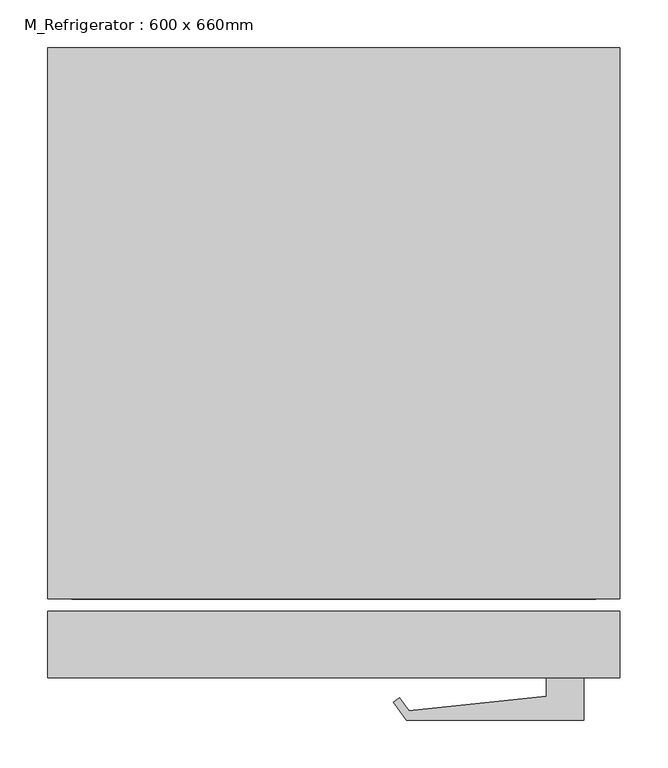
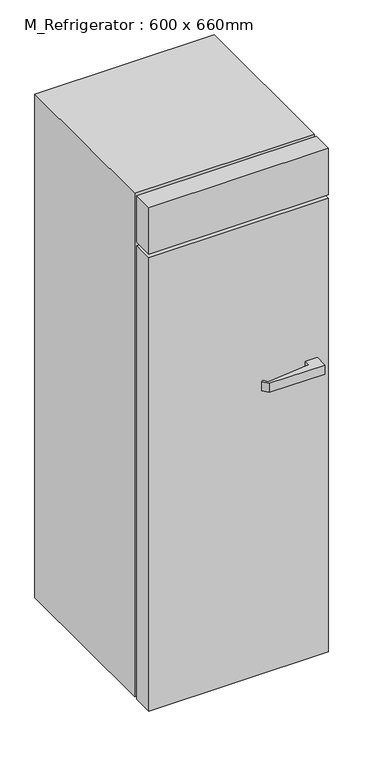
"""IFC4 building model written with IfcOpenShell, lengths in millimetres: proxy geometry, M_Refrigerator : 600 x 660mm."""

from ifc_helpers import new_model, si_unit, point, frame, frame_2d, origin, origin_with_axes, place, context, project, spatial, polyline, circle_curve, trimmed, segment, composite_curve, outline, extrude, source, transform, mapped, element, save


def m_refrigerator_600_x_660mm_a466bf94(model_context):
    return source(origin(), model_context, "Body", "SweptSolid", [
        extrude(outline(polyline([(208.0988574, -408.1036861), (22.3988574, -408.1036861), (8.7240737, -389.5368406), (15.2273026, -384.7471068), (25.1756383, -398.2543926), (168.9242419, -383.0358618), (168.9242419, -363.7849098), (208.0988574, -363.7849098), (208.0988574, -408.1036861)])), frame((0.0, 0.0, 1071.927792), z_axis=(0.0, 0.0, 1.0), x_axis=(1.0, 0.0, 0.0)), (0.0, 0.0, 1.0), 31.75),
        extrude(outline(composite_curve([segment(trimmed(circle_curve(frame_2d((-271.2511426, 220.0150902)), 25.4), [point((-296.6511426, 220.0150902))], [point((-245.8511426, 220.0150902))], False, "CARTESIAN"), True, "CONTINUOUS"), segment(trimmed(circle_curve(frame_2d((-271.2511426, 220.0150902)), 25.4), [point((-245.8511426, 220.0150902))], [point((-296.6511426, 220.0150902))], False, "CARTESIAN"), True, "CONTINUOUS")], self_intersect=False)), origin_with_axes(), (0.0, 0.0, 1.0), 50.8),
        extrude(outline(composite_curve([segment(trimmed(circle_curve(frame_2d((163.6488574, 220.0150902)), 25.4), [point((138.2488574, 220.0150902))], [point((189.0488574, 220.0150902))], False, "CARTESIAN"), True, "CONTINUOUS"), segment(trimmed(circle_curve(frame_2d((163.6488574, 220.0150902)), 25.4), [point((189.0488574, 220.0150902))], [point((138.2488574, 220.0150902))], False, "CARTESIAN"), True, "CONTINUOUS")], self_intersect=False)), origin_with_axes(), (0.0, 0.0, 1.0), 50.8),
        extrude(outline(composite_curve([segment(trimmed(circle_curve(frame_2d((-271.2511426, -236.7849098)), 25.4), [point((-296.6511426, -236.7849098))], [point((-245.8511426, -236.7849098))], False, "CARTESIAN"), True, "CONTINUOUS"), segment(trimmed(circle_curve(frame_2d((-271.2511426, -236.7849098)), 25.4), [point((-245.8511426, -236.7849098))], [point((-296.6511426, -236.7849098))], False, "CARTESIAN"), True, "CONTINUOUS")], self_intersect=False)), origin_with_axes(), (0.0, 0.0, 1.0), 50.8),
        extrude(outline(composite_curve([segment(trimmed(circle_curve(frame_2d((163.6488574, -236.7849098)), 25.4), [point((138.2488574, -236.7849098))], [point((189.0488574, -236.7849098))], False, "CARTESIAN"), True, "CONTINUOUS"), segment(trimmed(circle_curve(frame_2d((163.6488574, -236.7849098)), 25.4), [point((189.0488574, -236.7849098))], [point((138.2488574, -236.7849098))], False, "CARTESIAN"), True, "CONTINUOUS")], self_intersect=False)), origin_with_axes(), (0.0, 0.0, 1.0), 50.8),
        extrude(outline(polyline([(246.1988574, -363.7849098), (-353.8011426, -363.7849098), (-353.8011426, -293.9349098), (246.1988574, -293.9349098), (246.1988574, -363.7849098)])), frame((0.0, 0.0, 50.8), z_axis=(0.0, 0.0, 1.0), x_axis=(1.0, 0.0, 0.0)), (0.0, 0.0, 1.0), 1601.4),
        extrude(outline(polyline([(246.1988574, -363.7849098), (-353.8011426, -363.7849098), (-353.8011426, -293.9349098), (246.1988574, -293.9349098), (246.1988574, -363.7849098)])), frame((0.0, 0.0, 1664.9), z_axis=(0.0, 0.0, 1.0), x_axis=(1.0, 0.0, 0.0)), (0.0, 0.0, 1.0), 165.1),
        extrude(outline(polyline([(220.7988574, 270.8150902), (-328.4011426, 270.8150902), (-328.4011426, 296.2150902), (220.7988574, 296.2150902), (220.7988574, 270.8150902)])), frame((0.0, 0.0, 152.4), z_axis=(0.0, 0.0, 1.0), x_axis=(1.0, 0.0, 0.0)), (0.0, 0.0, 1.0), 1652.2),
        extrude(outline(polyline([(1830.0, 246.1988574), (1830.0, -353.8011426), (50.8, -353.8011426), (50.8, 246.1988574), (1830.0, 246.1988574)]), holes=[polyline([(1626.8, 220.7988574), (431.8, 220.7988574), (431.8, -328.4011426), (1626.8, -328.4011426), (1626.8, 220.7988574)])]), frame((0.0, -281.2349098, 0.0), z_axis=(0.0, 1.0, 0.0), x_axis=(0.0, 0.0, 1.0)), (0.0, 0.0, 1.0), 577.45),
    ])


if __name__ == "__main__":
    model = new_model("IFC4")
    model_context = context("Model", 3, world=origin())
    ifc_project = project(units=[si_unit("LENGTHUNIT", "METRE", prefix="MILLI")], contexts=[model_context])
    site = spatial("IfcSite", under=ifc_project)
    building = spatial("IfcBuilding", under=site)
    placement = place(None, origin())
    m_refrigerator_600_x_660mm_shape = m_refrigerator_600_x_660mm_a466bf94(model_context)
    element("IfcBuildingElementProxy", 1, Name="M_Refrigerator : 600 x 660mm", ObjectType="M_Refrigerator : 600 x 660mm", at=placement, inside=building, context=model_context, shape_type="MappedRepresentation", body=[
        mapped(m_refrigerator_600_x_660mm_shape, transform((0.0, 0.0, 0.0), x_axis=(1.0, 0.0, 0.0), y_axis=(0.0, 1.0, 0.0), z_axis=(0.0, 0.0, 1.0))),
    ])
    save(model, "model.ifc")

# Revit data of these elements
# Type "M_Refrigerator : 600 x 660mm"
#   Label = "REF."
#   Depth = 2' - 1.98425"
#   Height = 6' - 0.04724"
#   Width = 1' - 11.62205"
#   Material = Steel, Paint Finish, Ivory, Matte
#   Description = (empty or 0)
#   Default Elevation = 0
# Element 1 (IfcBuildingElementProxy, "M_Refrigerator : 600 x 660mm")
#   Materials on its faces: "Steel, Paint Finish, Ivory, Matte", "Steel, Chrome Plated"
# Materials
#   "Steel, Paint Finish, Ivory, Matte": class "Metal", colour RGB 247 247 239, transparency 0, Description = "Steel, paint finish, ivory, matte", Cost = 0
#   "Steel, Chrome Plated": class "Metal", colour RGB 244 244 244, transparency 0, Description = "Chromiuim plated steel", Cost = 0
